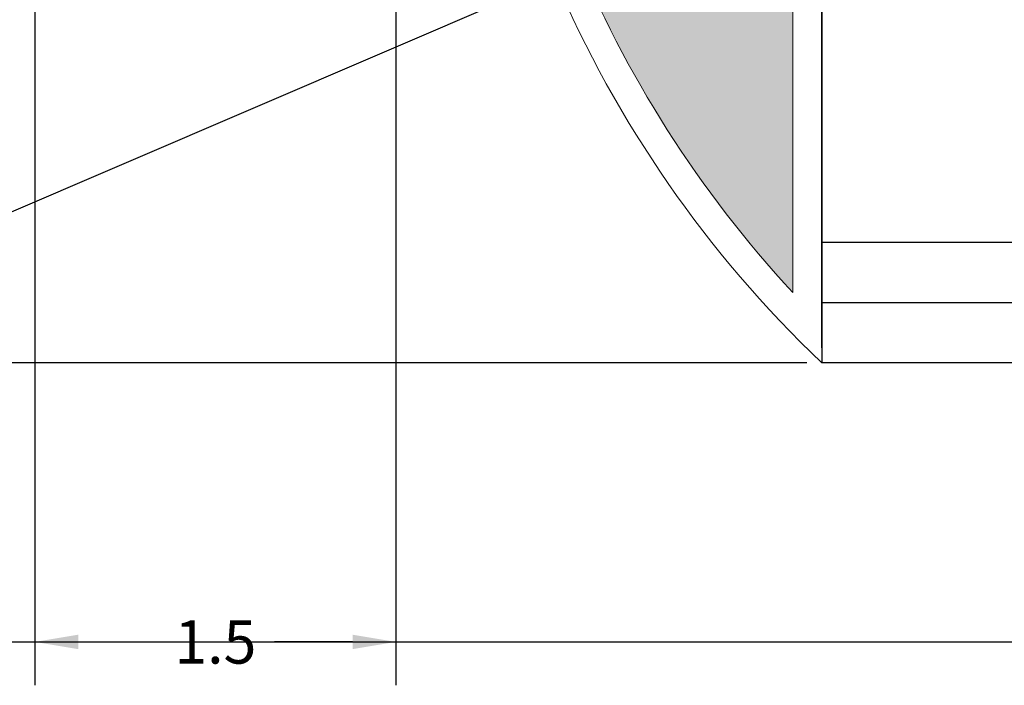
# Model space of a CAD drawing. Units: metres. Extents: x 4298.5 to 4325.2, y 2075 to 2095.8.
# Tile 3 of 35: x 4305.8 to 4309.9, y 2075 to 2077.8. Entities that reach past the tile are written whole.
import ezdxf

# ---------------------------------------------------------------- set-up
doc = ezdxf.new("R2010")
doc.units = ezdxf.units.M
for name, color, linetype, lineweight in [('A-ANNO-DIMS', 2, 'Continuous', 18), ('A-FLOR-STRS', 7, 'Continuous', 25), ('L-PLNT-BEDS', 94, 'Continuous', 18), ('L-PLNT-BEDS-PATT', 252, 'Continuous', 13)]:
    doc.layers.add(name, color=color, linetype=linetype, lineweight=lineweight)
doc.styles.get("Standard").update_dxf_attribs({"font": 'arial.ttf'})
doc.dimstyles.get("Standard").update_dxf_attribs({"dimtxt": 0.18, "dimasz": 0.18, "dimexe": 0.18, "dimexo": 0.0625, "dimgap": 0.09, "dimtad": 0, "dimtih": 1, "dimtoh": 1, "dimdec": 4, "dimzin": 0, "dimdsep": 46, "dimtxsty": 'Standard', "dimcen": 0.09, "dimadec": 0, "dimazin": 0, "dimtfac": 1, "dimtdec": 4, "dimtofl": 0, "dimtmove": 0, "dimatfit": 3, "dimfxl": 1, "dimtolj": 1, "dimtzin": 0, "dimarcsym": 0})

# ---------------------------------------------------------------- blocks, each defined once
blk = doc.blocks.new('*D47')
at = {"layer": 'A-ANNO-DIMS', "color": 0, "lineweight": -2, "transparency": 16777216}
for p, q in [((4300.4306, 2084.4956), (4300.4306, 2074.9896)), ((4322.8106, 2084.4956), (4322.8106, 2074.9896)), ((4300.6106, 2075.1696), (4311.2252, 2075.1696)), ((4322.6306, 2075.1696), (4312.016, 2075.1696))]:
    blk.add_line(p, q, dxfattribs=at)
at = {"layer": 'A-ANNO-DIMS', "color": 0, "transparency": 16777216}
for points in [[(4300.6106, 2075.1996), (4300.6106, 2075.1396), (4300.4306, 2075.1696)], [(4322.6306, 2075.1996), (4322.6306, 2075.1396), (4322.8106, 2075.1696)]]:
    blk.add_solid(points, dxfattribs=at)
at = {"layer": 'Defpoints', "color": 0, "transparency": 16777216}
for p in [(4300.4306, 2084.5581), (4322.8106, 2084.5581), (4322.8106, 2075.1696)]:
    blk.add_point(p, dxfattribs=at)
at = {"layer": 'A-ANNO-DIMS', "color": 0, "transparency": 16777216, "insert": (4311.6206, 2075.1696), "char_height": 0.18, "attachment_point": 5}
blk.add_mtext('\\A1;22.38', dxfattribs=at)
blk = doc.blocks.new('*D53')
at = {"layer": 'A-ANNO-DIMS', "color": 0, "lineweight": -2, "transparency": 16777216}
for p, q in [((4309.1606, 2076.3906), (4309.1606, 2095.8166)), ((4316.8106, 2076.3906), (4316.8106, 2095.8166)), ((4309.3406, 2095.6366), (4312.6619, 2095.6366)), ((4316.6306, 2095.6366), (4313.3093, 2095.6366))]:
    blk.add_line(p, q, dxfattribs=at)
at = {"layer": 'A-ANNO-DIMS', "color": 0, "transparency": 16777216}
for points in [[(4309.3406, 2095.6666), (4309.3406, 2095.6066), (4309.1606, 2095.6366)], [(4316.6306, 2095.6666), (4316.6306, 2095.6066), (4316.8106, 2095.6366)]]:
    blk.add_solid(points, dxfattribs=at)
at = {"layer": 'Defpoints', "color": 0, "transparency": 16777216}
for p in [(4316.8106, 2095.6366), (4309.1606, 2076.3281), (4316.8106, 2076.3281)]:
    blk.add_point(p, dxfattribs=at)
at = {"layer": 'A-ANNO-DIMS', "color": 0, "transparency": 16777216, "insert": (4312.9856, 2095.6366), "char_height": 0.18, "attachment_point": 5}
blk.add_mtext('\\A1;7.65', dxfattribs=at)
blk = doc.blocks.new('*D54')
at = {"layer": 'A-ANNO-DIMS', "color": 0, "lineweight": -2, "transparency": 16777216}
for p, q in [((4305.5981, 2079.8281), (4299.0921, 2079.8281)), ((4299.2721, 2079.6481), (4299.2721, 2078.26)), ((4299.2721, 2076.5081), (4299.2721, 2077.8961)), ((4309.0981, 2076.3281), (4299.0921, 2076.3281))]:
    blk.add_line(p, q, dxfattribs=at)
at = {"layer": 'A-ANNO-DIMS', "color": 0, "transparency": 16777216}
for points in [[(4299.2421, 2079.6481), (4299.3021, 2079.6481), (4299.2721, 2079.8281)], [(4299.2421, 2076.5081), (4299.3021, 2076.5081), (4299.2721, 2076.3281)]]:
    blk.add_solid(points, dxfattribs=at)
at = {"layer": 'Defpoints', "color": 0, "transparency": 16777216}
for p in [(4305.6606, 2079.8281), (4299.2721, 2076.3281), (4309.1606, 2076.3281)]:
    blk.add_point(p, dxfattribs=at)
at = {"layer": 'A-ANNO-DIMS', "color": 0, "transparency": 16777216, "insert": (4299.2721, 2078.0781), "char_height": 0.18, "attachment_point": 5}
blk.add_mtext('\\A1;3.5', dxfattribs=at)
blk = doc.blocks.new('*D59')
at = {"layer": 'A-ANNO-DIMS', "color": 0, "lineweight": -2, "transparency": 16777216}
for p, q in [((4305.8906, 2079.9956), (4305.8906, 2074.9896)), ((4307.3906, 2079.9956), (4307.3906, 2074.9896)), ((4306.0706, 2075.1696), (4306.3945, 2075.1696)), ((4307.2106, 2075.1696), (4306.8866, 2075.1696))]:
    blk.add_line(p, q, dxfattribs=at)
at = {"layer": 'A-ANNO-DIMS', "color": 0, "transparency": 16777216}
for points in [[(4306.0706, 2075.1996), (4306.0706, 2075.1396), (4305.8906, 2075.1696)], [(4307.2106, 2075.1996), (4307.2106, 2075.1396), (4307.3906, 2075.1696)]]:
    blk.add_solid(points, dxfattribs=at)
at = {"layer": 'Defpoints', "color": 0, "transparency": 16777216}
for p in [(4305.8906, 2080.0581), (4307.3906, 2080.0581), (4307.3906, 2075.1696)]:
    blk.add_point(p, dxfattribs=at)
at = {"layer": 'A-ANNO-DIMS', "color": 0, "transparency": 16777216, "insert": (4306.6406, 2075.1696), "char_height": 0.18, "attachment_point": 5}
blk.add_mtext('\\A1;1.5', dxfattribs=at)
blk = doc.blocks.new('*D78')
at = {"layer": 'A-ANNO-DIMS', "color": 0, "lineweight": -2, "transparency": 16777216}
for p, q in [((4312.4969, 2079.7393), (4312.4969, 2079.9193)), ((4312.4069, 2079.8293), (4312.5869, 2079.8293)), ((4305.3847, 2076.7806), (4307.8863, 2077.853)), ((4305.2047, 2076.7806), (4305.3847, 2076.7806))]:
    blk.add_line(p, q, dxfattribs=at)
at = {"layer": 'A-ANNO-DIMS', "color": 0, "transparency": 16777216}
blk.add_solid([(4307.8745, 2077.8806), (4307.8981, 2077.8254), (4308.0518, 2077.9239)], dxfattribs=at)
at = {"layer": 'Defpoints', "color": 0, "transparency": 16777216}
for p in [(4312.4969, 2079.8293), (4308.0518, 2077.9239)]:
    blk.add_point(p, dxfattribs=at)
at = {"layer": 'A-ANNO-DIMS', "color": 0, "transparency": 16777216, "insert": (4304.53, 2076.7806), "char_height": 0.18, "attachment_point": 5}
blk.add_mtext('\\A1;2X R4.836', dxfattribs=at)

msp = doc.modelspace()

# ---------------------------------------------------------------- hatches: boundary and pattern name
at = {"layer": 'L-PLNT-BEDS-PATT'}
h = msp.add_hatch(dxfattribs=at)
h.set_pattern_fill('TRIANG', color=256, scale=0.02)
h.paths.add_polyline_path([(4309.0406, 2079.7081), (4307.7821, 2079.7081, 0.182638), (4309.0406, 2076.6204)])
h.paths.add_polyline_path([(4318.189, 2079.7081), (4316.9306, 2079.7081), (4316.9306, 2076.6204, 0.182638)])

# ---------------------------------------------------------------- linework, layer by layer
at = {"layer": 'A-FLOR-STRS'}
for p, q in [((4309.1606, 2079.8281), (4309.1606, 2076.3281)), ((4316.8106, 2076.8281), (4309.1606, 2076.8281)), ((4316.8106, 2076.5781), (4309.1606, 2076.5781)), ((4316.8106, 2076.3281), (4309.1606, 2076.3281))]:
    msp.add_line(p, q, dxfattribs=at)
at = {"layer": 'L-PLNT-BEDS'}
msp.add_line((4309.0406, 2079.7081), (4309.0406, 2076.6204), dxfattribs=at)
for radius, start, end in [(4.8363, 180.0152, 226.382), (4.7163, 181.4735, 222.8748)]:
    msp.add_arc((4312.4969, 2079.8293), radius, start, end, dxfattribs=at)

# ---------------------------------------------------------------- dimensions: what is measured, and where the dimension line sits
at = {"layer": 'A-ANNO-DIMS'}
for base, p1, p2, override, picture, middle in [((4316.8106, 2095.6366), (4309.1606, 2076.3281), (4316.8106, 2076.3281), {"dimdec": 2, "dimlfac": 1, "dimrnd": 0, "dimzin": 0, "dimdsep": 46, "dimlunit": 2}, '*D53', (4312.9856, 2095.6366)), ((4322.8106, 2075.1696), (4300.4306, 2084.5581), (4322.8106, 2084.5581), {"dimdec": 2, "dimlfac": 1, "dimrnd": 0, "dimzin": 0, "dimdsep": 46, "dimlunit": 2}, '*D47', (4311.6206, 2075.1696)), ((4307.3906, 2075.1696), (4305.8906, 2080.0581), (4307.3906, 2080.0581), {"dimdec": 1, "dimlfac": 1, "dimrnd": 0, "dimzin": 0, "dimdsep": 46, "dimlunit": 2}, '*D59', (4306.6406, 2075.1696))]:
    dim = msp.add_linear_dim(base=base, p1=p1, p2=p2, dimstyle='Standard', override=override, dxfattribs=at)
    dim.commit()
    dim.dimension.update_dxf_attribs({"geometry": picture, "text_midpoint": middle})
dim = msp.add_radius_dim(center=(4312.4969, 2079.8293), mpoint=(4308.0518, 2077.9239), text='2X <>', dimstyle='Standard', override={"dimdec": 3, "dimlfac": 1, "dimrnd": 0, "dimzin": 0, "dimdsep": 46, "dimlunit": 2}, dxfattribs=at)
dim.commit()
dim.dimension.update_dxf_attribs({"geometry": '*D78', "text_midpoint": (4304.53, 2076.7806), "dimtype": 164})
dim = msp.add_linear_dim(base=(4299.2721, 2076.3281), p1=(4305.6606, 2079.8281), p2=(4309.1606, 2076.3281), angle=90, dimstyle='Standard', override={"dimdec": 1, "dimlfac": 1, "dimrnd": 0, "dimzin": 0, "dimdsep": 46, "dimlunit": 2}, dxfattribs=at)
dim.commit()
dim.dimension.update_dxf_attribs({"geometry": '*D54', "text_midpoint": (4299.2721, 2078.0781)})

doc.saveas('drawing.dxf')
